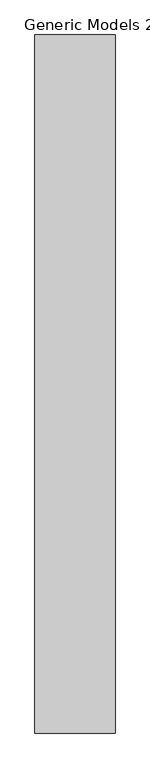
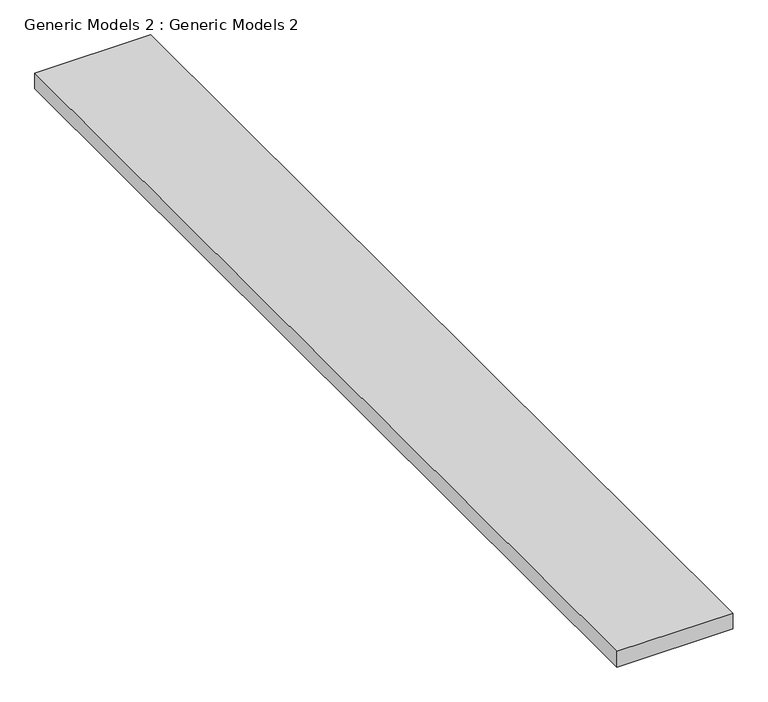
"""IFC4 building model written with IfcOpenShell, lengths in millimetres: proxy geometry, Generic Models 2 : Generic Models 2."""

from ifc_helpers import new_model, si_unit, frame, origin, place, context, project, spatial, polyline, outline, extrude, source, transform, mapped, element, save


def generic_models_2_generic_models_2_8d9d6b08(model_context):
    return source(origin(), model_context, "Body", "SweptSolid", [
        extrude(outline(polyline([(12941.3, 17386.3), (12941.3, -1130.3), (10816.1582871, -1130.3), (10816.1582871, 17386.3), (12941.3, 17386.3)])), frame((0.0, 0.0, -76.2), z_axis=(0.0, 0.0, 1.0), x_axis=(1.0, 0.0, 0.0)), (0.0, 0.0, 1.0), 304.8),
    ])


if __name__ == "__main__":
    model = new_model("IFC4")
    model_context = context("Model", 3, world=origin())
    ifc_project = project(units=[si_unit("LENGTHUNIT", "METRE", prefix="MILLI")], contexts=[model_context])
    site = spatial("IfcSite", under=ifc_project)
    building = spatial("IfcBuilding", under=site)
    placement = place(None, origin())
    generic_models_2_generic_models_2_shape = generic_models_2_generic_models_2_8d9d6b08(model_context)
    element("IfcBuildingElementProxy", 1, Name="Generic Models 2 : Generic Models 2", ObjectType="Generic Models 2 : Generic Models 2", at=placement, inside=building, context=model_context, shape_type="MappedRepresentation", body=[
        mapped(generic_models_2_generic_models_2_shape, transform((0.0, 0.0, 0.0), x_axis=(1.0, 0.0, 0.0), y_axis=(0.0, 1.0, 0.0), z_axis=(0.0, 0.0, 1.0))),
    ])
    save(model, "model.ifc")
